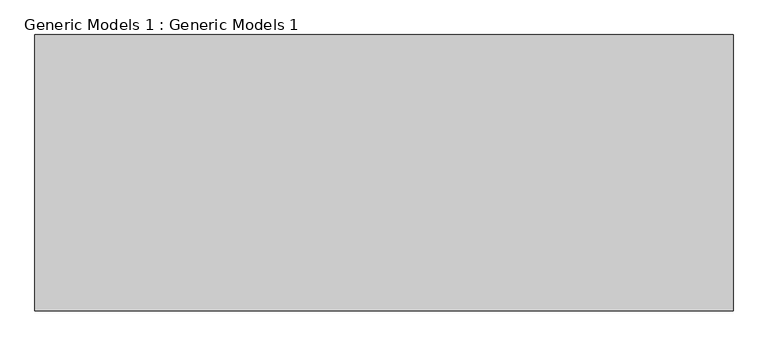
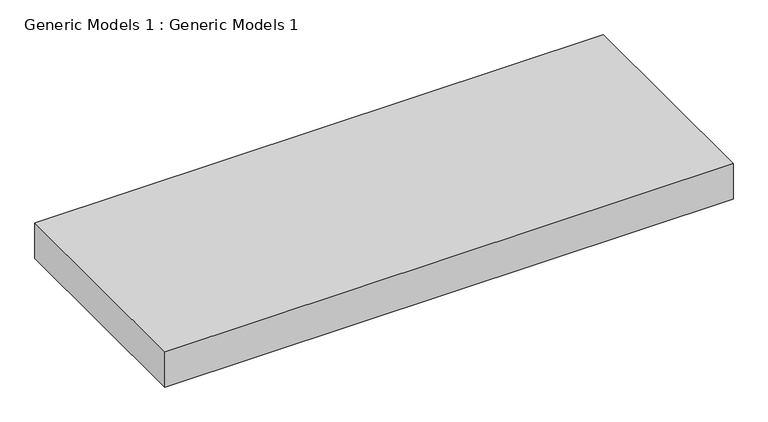
"""IFC4 building model written with IfcOpenShell, lengths in millimetres: proxy geometry, Generic Models 1 : Generic Models 1."""

from ifc_helpers import new_model, si_unit, frame, origin, place, context, project, spatial, polyline, outline, extrude, source, transform, mapped, element, save


def generic_models_1_generic_models_1_0485f0a6(model_context):
    return source(origin(), model_context, "Body", "SweptSolid", [
        extrude(outline(polyline([(-29652.0588466, 5414.3256148), (-31963.4588466, 5414.3256148), (-31963.4588466, 6328.7256148), (-29652.0588466, 6328.7256148), (-29652.0588466, 5414.3256148)])), frame((0.0, 0.0, 2309.7077474), z_axis=(0.0, 0.0, 1.0), x_axis=(1.0, 0.0, 0.0)), (0.0, 0.0, 1.0), 152.4),
    ])


if __name__ == "__main__":
    model = new_model("IFC4")
    model_context = context("Model", 3, world=origin())
    ifc_project = project(units=[si_unit("LENGTHUNIT", "METRE", prefix="MILLI")], contexts=[model_context])
    site = spatial("IfcSite", under=ifc_project)
    building = spatial("IfcBuilding", under=site)
    placement = place(None, origin())
    generic_models_1_generic_models_1_shape = generic_models_1_generic_models_1_0485f0a6(model_context)
    element("IfcBuildingElementProxy", 1, Name="Generic Models 1 : Generic Models 1", ObjectType="Generic Models 1 : Generic Models 1", at=placement, inside=building, context=model_context, shape_type="MappedRepresentation", body=[
        mapped(generic_models_1_generic_models_1_shape, transform((0.0, 0.0, 0.0), x_axis=(1.0, 0.0, 0.0), y_axis=(0.0, 1.0, 0.0), z_axis=(0.0, 0.0, 1.0))),
    ])
    save(model, "model.ifc")
